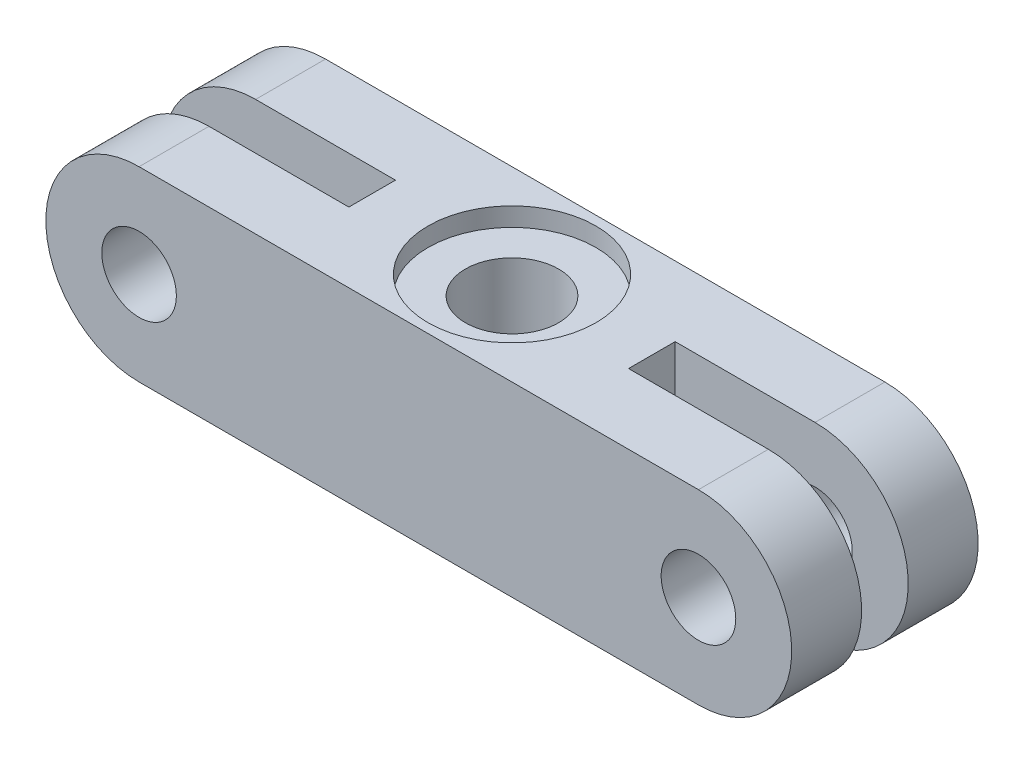
ISO-10303-21;
HEADER;
FILE_DESCRIPTION(('STEP AP214'),'2;1');
FILE_NAME('part.step','',(''),(''),'','','');
FILE_SCHEMA(('AUTOMOTIVE_DESIGN { 1 0 10303 214 1 1 1 1 }'));
ENDSEC;
DATA;
#1=APPLICATION_CONTEXT('core data for automotive mechanical design processes');
#2=APPLICATION_PROTOCOL_DEFINITION('international standard','automotive_design',2000,#1);
#3=PRODUCT_CONTEXT('',#1,'mechanical');
#4=PRODUCT('Part','Part','',(#3));
#5=PRODUCT_RELATED_PRODUCT_CATEGORY('part','',(#4));
#6=PRODUCT_DEFINITION_FORMATION('','',#4);
#7=PRODUCT_DEFINITION_CONTEXT('part definition',#1,'design');
#8=PRODUCT_DEFINITION('design','',#6,#7);
#9=PRODUCT_DEFINITION_SHAPE('','',#8);
#10=(LENGTH_UNIT() NAMED_UNIT(*) SI_UNIT(.MILLI.,.METRE.));
#11=(NAMED_UNIT(*) PLANE_ANGLE_UNIT() SI_UNIT($,.RADIAN.));
#12=(NAMED_UNIT(*) SI_UNIT($,.STERADIAN.) SOLID_ANGLE_UNIT());
#13=UNCERTAINTY_MEASURE_WITH_UNIT(LENGTH_MEASURE(1.E-05),#10,'distance_accuracy_value','');
#14=(GEOMETRIC_REPRESENTATION_CONTEXT(3) GLOBAL_UNCERTAINTY_ASSIGNED_CONTEXT((#13)) GLOBAL_UNIT_ASSIGNED_CONTEXT((#10,
#11,#12)) REPRESENTATION_CONTEXT('',''));
#15=CARTESIAN_POINT('',(0.,0.,0.));
#16=DIRECTION('',(0.,0.,1.));
#17=DIRECTION('',(1.,0.,0.));
#18=AXIS2_PLACEMENT_3D('',#15,#16,#17);
#19=CARTESIAN_POINT('',(0.,-10.,0.));
#20=DIRECTION('',(0.,1.,0.));
#21=DIRECTION('',(-1.,0.,0.));
#22=AXIS2_PLACEMENT_3D('',#19,#20,#21);
#23=CYLINDRICAL_SURFACE('',#22,5.);
#24=CARTESIAN_POINT('',(0.,-10.,0.));
#25=DIRECTION('',(0.,1.,0.));
#26=DIRECTION('',(-1.,0.,0.));
#27=AXIS2_PLACEMENT_3D('',#24,#25,#26);
#28=CIRCLE('',#27,5.);
#29=CARTESIAN_POINT('',(-5.,-10.,0.));
#30=VERTEX_POINT('',#29);
#31=EDGE_CURVE('E158',#30,#30,#28,.T.);
#32=ORIENTED_EDGE('',*,*,#31,.F.);
#33=EDGE_LOOP('',(#32));
#34=FACE_BOUND('',#33,.T.);
#35=CARTESIAN_POINT('',(0.,8.00000000000001,0.));
#36=DIRECTION('',(0.,1.,0.));
#37=DIRECTION('',(-1.,0.,0.));
#38=AXIS2_PLACEMENT_3D('',#35,#36,#37);
#39=CIRCLE('',#38,5.);
#40=CARTESIAN_POINT('',(-5.,8.00000000000001,0.));
#41=VERTEX_POINT('',#40);
#42=EDGE_CURVE('E44',#41,#41,#39,.F.);
#43=ORIENTED_EDGE('',*,*,#42,.F.);
#44=EDGE_LOOP('',(#43));
#45=FACE_BOUND('',#44,.T.);
#46=ADVANCED_FACE('F41',(#34,#45),#23,.F.);
#47=CARTESIAN_POINT('',(-30.,0.,10.));
#48=DIRECTION('',(0.,0.,-1.));
#49=DIRECTION('',(-1.,0.,0.));
#50=AXIS2_PLACEMENT_3D('',#47,#48,#49);
#51=CYLINDRICAL_SURFACE('',#50,10.);
#52=CARTESIAN_POINT('',(-30.,0.,-2.5));
#53=DIRECTION('',(0.,0.,-1.));
#54=DIRECTION('',(-1.,0.,0.));
#55=AXIS2_PLACEMENT_3D('',#52,#53,#54);
#56=CIRCLE('',#55,10.);
#57=CARTESIAN_POINT('',(-30.,-10.,-2.5));
#58=VERTEX_POINT('',#57);
#59=CARTESIAN_POINT('',(-30.,10.,-2.5));
#60=VERTEX_POINT('',#59);
#61=EDGE_CURVE('E194',#58,#60,#56,.T.);
#62=ORIENTED_EDGE('',*,*,#61,.T.);
#63=DIRECTION('',(0.,0.,-1.));
#64=VECTOR('',#63,1.);
#65=CARTESIAN_POINT('',(-30.,10.,10.));
#66=LINE('',#65,#64);
#67=CARTESIAN_POINT('',(-30.,10.,-10.));
#68=VERTEX_POINT('',#67);
#69=EDGE_CURVE('E217',#60,#68,#66,.T.);
#70=ORIENTED_EDGE('',*,*,#69,.T.);
#71=CARTESIAN_POINT('',(-30.,0.,-10.));
#72=DIRECTION('',(0.,0.,1.));
#73=DIRECTION('',(1.,0.,0.));
#74=AXIS2_PLACEMENT_3D('',#71,#72,#73);
#75=CIRCLE('',#74,10.);
#76=CARTESIAN_POINT('',(-30.,-10.,-10.));
#77=VERTEX_POINT('',#76);
#78=EDGE_CURVE('E202',#68,#77,#75,.T.);
#79=ORIENTED_EDGE('',*,*,#78,.T.);
#80=DIRECTION('',(0.,0.,-1.));
#81=VECTOR('',#80,1.);
#82=CARTESIAN_POINT('',(-30.,-10.,10.));
#83=LINE('',#82,#81);
#84=EDGE_CURVE('E49',#58,#77,#83,.T.);
#85=ORIENTED_EDGE('',*,*,#84,.F.);
#86=EDGE_LOOP('',(#62,#70,#79,#85));
#87=FACE_BOUND('',#86,.T.);
#88=ADVANCED_FACE('F283',(#87),#51,.T.);
#89=CARTESIAN_POINT('',(30.,0.,10.));
#90=DIRECTION('',(0.,0.,-1.));
#91=DIRECTION('',(-1.,0.,0.));
#92=AXIS2_PLACEMENT_3D('',#89,#90,#91);
#93=CYLINDRICAL_SURFACE('',#92,10.);
#94=DIRECTION('',(0.,0.,-1.));
#95=VECTOR('',#94,1.);
#96=CARTESIAN_POINT('',(30.,10.,10.));
#97=LINE('',#96,#95);
#98=CARTESIAN_POINT('',(30.,10.,-2.5));
#99=VERTEX_POINT('',#98);
#100=CARTESIAN_POINT('',(30.,10.,-10.));
#101=VERTEX_POINT('',#100);
#102=EDGE_CURVE('E235',#99,#101,#97,.T.);
#103=ORIENTED_EDGE('',*,*,#102,.F.);
#104=CARTESIAN_POINT('',(30.,0.,-2.5));
#105=DIRECTION('',(0.,0.,-1.));
#106=DIRECTION('',(-1.,0.,0.));
#107=AXIS2_PLACEMENT_3D('',#104,#105,#106);
#108=CIRCLE('',#107,10.);
#109=CARTESIAN_POINT('',(30.,-10.,-2.5));
#110=VERTEX_POINT('',#109);
#111=EDGE_CURVE('E189',#99,#110,#108,.T.);
#112=ORIENTED_EDGE('',*,*,#111,.T.);
#113=DIRECTION('',(0.,0.,-1.));
#114=VECTOR('',#113,1.);
#115=CARTESIAN_POINT('',(30.,-9.99999999999999,10.));
#116=LINE('',#115,#114);
#117=CARTESIAN_POINT('',(30.,-9.99999999999999,-10.));
#118=VERTEX_POINT('',#117);
#119=EDGE_CURVE('E237',#110,#118,#116,.T.);
#120=ORIENTED_EDGE('',*,*,#119,.T.);
#121=CARTESIAN_POINT('',(30.,0.,-10.));
#122=DIRECTION('',(0.,0.,1.));
#123=DIRECTION('',(1.,0.,0.));
#124=AXIS2_PLACEMENT_3D('',#121,#122,#123);
#125=CIRCLE('',#124,10.);
#126=EDGE_CURVE('E221',#118,#101,#125,.T.);
#127=ORIENTED_EDGE('',*,*,#126,.T.);
#128=EDGE_LOOP('',(#103,#112,#120,#127));
#129=FACE_BOUND('',#128,.T.);
#130=ADVANCED_FACE('F254',(#129),#93,.T.);
#131=CARTESIAN_POINT('',(-30.,0.,10.));
#132=DIRECTION('',(0.,0.,-1.));
#133=DIRECTION('',(-1.,0.,0.));
#134=AXIS2_PLACEMENT_3D('',#131,#132,#133);
#135=CYLINDRICAL_SURFACE('',#134,4.);
#136=CARTESIAN_POINT('',(-30.,0.,-2.5));
#137=DIRECTION('',(0.,0.,-1.));
#138=DIRECTION('',(-1.,0.,0.));
#139=AXIS2_PLACEMENT_3D('',#136,#137,#138);
#140=CIRCLE('',#139,4.);
#141=CARTESIAN_POINT('',(-34.,0.,-2.5));
#142=VERTEX_POINT('',#141);
#143=EDGE_CURVE('E195',#142,#142,#140,.T.);
#144=ORIENTED_EDGE('',*,*,#143,.F.);
#145=EDGE_LOOP('',(#144));
#146=FACE_BOUND('',#145,.T.);
#147=CARTESIAN_POINT('',(-30.,0.,-10.));
#148=DIRECTION('',(0.,0.,1.));
#149=DIRECTION('',(1.,0.,0.));
#150=AXIS2_PLACEMENT_3D('',#147,#148,#149);
#151=CIRCLE('',#150,4.);
#152=CARTESIAN_POINT('',(-26.,0.,-10.));
#153=VERTEX_POINT('',#152);
#154=EDGE_CURVE('E200',#153,#153,#151,.T.);
#155=ORIENTED_EDGE('',*,*,#154,.F.);
#156=EDGE_LOOP('',(#155));
#157=FACE_BOUND('',#156,.T.);
#158=ADVANCED_FACE('F253',(#146,#157),#135,.F.);
#159=CARTESIAN_POINT('',(30.,0.,10.));
#160=DIRECTION('',(0.,0.,-1.));
#161=DIRECTION('',(-1.,0.,0.));
#162=AXIS2_PLACEMENT_3D('',#159,#160,#161);
#163=CYLINDRICAL_SURFACE('',#162,4.00000000000001);
#164=CARTESIAN_POINT('',(30.,0.,-2.5));
#165=DIRECTION('',(0.,0.,-1.));
#166=DIRECTION('',(-1.,0.,0.));
#167=AXIS2_PLACEMENT_3D('',#164,#165,#166);
#168=CIRCLE('',#167,4.00000000000001);
#169=CARTESIAN_POINT('',(26.,0.,-2.5));
#170=VERTEX_POINT('',#169);
#171=EDGE_CURVE('E187',#170,#170,#168,.T.);
#172=ORIENTED_EDGE('',*,*,#171,.F.);
#173=EDGE_LOOP('',(#172));
#174=FACE_BOUND('',#173,.T.);
#175=CARTESIAN_POINT('',(30.,0.,-10.));
#176=DIRECTION('',(0.,0.,1.));
#177=DIRECTION('',(1.,0.,0.));
#178=AXIS2_PLACEMENT_3D('',#175,#176,#177);
#179=CIRCLE('',#178,4.00000000000001);
#180=CARTESIAN_POINT('',(34.,0.,-10.));
#181=VERTEX_POINT('',#180);
#182=EDGE_CURVE('E193',#181,#181,#179,.T.);
#183=ORIENTED_EDGE('',*,*,#182,.F.);
#184=EDGE_LOOP('',(#183));
#185=FACE_BOUND('',#184,.T.);
#186=ADVANCED_FACE('F255',(#174,#185),#163,.F.);
#187=CARTESIAN_POINT('',(-30.,0.,10.));
#188=DIRECTION('',(0.,0.,1.));
#189=DIRECTION('',(1.,0.,0.));
#190=AXIS2_PLACEMENT_3D('',#187,#188,#189);
#191=PLANE('',#190);
#192=CARTESIAN_POINT('',(-30.,0.,10.));
#193=DIRECTION('',(0.,0.,1.));
#194=DIRECTION('',(1.,0.,0.));
#195=AXIS2_PLACEMENT_3D('',#192,#193,#194);
#196=CIRCLE('',#195,4.);
#197=CARTESIAN_POINT('',(-26.,0.,10.));
#198=VERTEX_POINT('',#197);
#199=EDGE_CURVE('E205',#198,#198,#196,.T.);
#200=ORIENTED_EDGE('',*,*,#199,.F.);
#201=EDGE_LOOP('',(#200));
#202=FACE_BOUND('',#201,.T.);
#203=CARTESIAN_POINT('',(-30.,0.,10.));
#204=DIRECTION('',(0.,0.,1.));
#205=DIRECTION('',(1.,0.,0.));
#206=AXIS2_PLACEMENT_3D('',#203,#204,#205);
#207=CIRCLE('',#206,10.);
#208=CARTESIAN_POINT('',(-30.,10.,10.));
#209=VERTEX_POINT('',#208);
#210=CARTESIAN_POINT('',(-30.,-10.,10.));
#211=VERTEX_POINT('',#210);
#212=EDGE_CURVE('E208',#209,#211,#207,.T.);
#213=ORIENTED_EDGE('',*,*,#212,.T.);
#214=DIRECTION('',(1.,0.,0.));
#215=VECTOR('',#214,1.);
#216=CARTESIAN_POINT('',(-30.,-10.,10.));
#217=LINE('',#216,#215);
#218=CARTESIAN_POINT('',(30.,-9.99999999999999,10.));
#219=VERTEX_POINT('',#218);
#220=EDGE_CURVE('E211',#211,#219,#217,.T.);
#221=ORIENTED_EDGE('',*,*,#220,.T.);
#222=CARTESIAN_POINT('',(30.,0.,10.));
#223=DIRECTION('',(0.,0.,1.));
#224=DIRECTION('',(1.,0.,0.));
#225=AXIS2_PLACEMENT_3D('',#222,#223,#224);
#226=CIRCLE('',#225,10.);
#227=CARTESIAN_POINT('',(30.,10.,10.));
#228=VERTEX_POINT('',#227);
#229=EDGE_CURVE('E212',#219,#228,#226,.T.);
#230=ORIENTED_EDGE('',*,*,#229,.T.);
#231=DIRECTION('',(-1.,0.,0.));
#232=VECTOR('',#231,1.);
#233=CARTESIAN_POINT('',(-30.,10.,10.));
#234=LINE('',#233,#232);
#235=EDGE_CURVE('E216',#228,#209,#234,.T.);
#236=ORIENTED_EDGE('',*,*,#235,.T.);
#237=EDGE_LOOP('',(#213,#221,#230,#236));
#238=FACE_BOUND('',#237,.T.);
#239=CARTESIAN_POINT('',(30.,0.,10.));
#240=DIRECTION('',(0.,0.,1.));
#241=DIRECTION('',(1.,0.,0.));
#242=AXIS2_PLACEMENT_3D('',#239,#240,#241);
#243=CIRCLE('',#242,4.00000000000001);
#244=CARTESIAN_POINT('',(34.,0.,10.));
#245=VERTEX_POINT('',#244);
#246=EDGE_CURVE('E198',#245,#245,#243,.T.);
#247=ORIENTED_EDGE('',*,*,#246,.F.);
#248=EDGE_LOOP('',(#247));
#249=FACE_BOUND('',#248,.T.);
#250=ADVANCED_FACE('F263',(#202,#238,#249),#191,.T.);
#251=CARTESIAN_POINT('',(-30.,0.,-10.));
#252=DIRECTION('',(0.,0.,1.));
#253=DIRECTION('',(1.,0.,0.));
#254=AXIS2_PLACEMENT_3D('',#251,#252,#253);
#255=PLANE('',#254);
#256=ORIENTED_EDGE('',*,*,#78,.F.);
#257=DIRECTION('',(-1.,0.,0.));
#258=VECTOR('',#257,1.);
#259=CARTESIAN_POINT('',(-30.,10.,-10.));
#260=LINE('',#259,#258);
#261=EDGE_CURVE('E215',#101,#68,#260,.T.);
#262=ORIENTED_EDGE('',*,*,#261,.F.);
#263=ORIENTED_EDGE('',*,*,#126,.F.);
#264=DIRECTION('',(1.,0.,0.));
#265=VECTOR('',#264,1.);
#266=CARTESIAN_POINT('',(-30.,-10.,-10.));
#267=LINE('',#266,#265);
#268=EDGE_CURVE('E222',#77,#118,#267,.T.);
#269=ORIENTED_EDGE('',*,*,#268,.F.);
#270=EDGE_LOOP('',(#256,#262,#263,#269));
#271=FACE_BOUND('',#270,.T.);
#272=ORIENTED_EDGE('',*,*,#154,.T.);
#273=EDGE_LOOP('',(#272));
#274=FACE_BOUND('',#273,.T.);
#275=ORIENTED_EDGE('',*,*,#182,.T.);
#276=EDGE_LOOP('',(#275));
#277=FACE_BOUND('',#276,.T.);
#278=ADVANCED_FACE('F257',(#271,#274,#277),#255,.F.);
#279=CARTESIAN_POINT('',(-30.,10.,2.5));
#280=VERTEX_POINT('',#279);
#281=EDGE_CURVE('E228',#209,#280,#66,.T.);
#282=ORIENTED_EDGE('',*,*,#281,.T.);
#283=CARTESIAN_POINT('',(-30.,0.,2.5));
#284=DIRECTION('',(0.,0.,1.));
#285=DIRECTION('',(1.,0.,0.));
#286=AXIS2_PLACEMENT_3D('',#283,#284,#285);
#287=CIRCLE('',#286,10.);
#288=CARTESIAN_POINT('',(-30.,-10.,2.5));
#289=VERTEX_POINT('',#288);
#290=EDGE_CURVE('E67',#280,#289,#287,.T.);
#291=ORIENTED_EDGE('',*,*,#290,.T.);
#292=EDGE_CURVE('E11',#211,#289,#83,.T.);
#293=ORIENTED_EDGE('',*,*,#292,.F.);
#294=ORIENTED_EDGE('',*,*,#212,.F.);
#295=EDGE_LOOP('',(#282,#291,#293,#294));
#296=FACE_BOUND('',#295,.T.);
#297=ADVANCED_FACE('F43',(#296),#51,.T.);
#298=CARTESIAN_POINT('',(-30.,-10.,10.));
#299=DIRECTION('',(0.,1.,0.));
#300=DIRECTION('',(-1.,0.,0.));
#301=AXIS2_PLACEMENT_3D('',#298,#299,#300);
#302=PLANE('',#301);
#303=ORIENTED_EDGE('',*,*,#31,.T.);
#304=EDGE_LOOP('',(#303));
#305=FACE_BOUND('',#304,.T.);
#306=DIRECTION('',(0.,0.,-1.));
#307=VECTOR('',#306,1.);
#308=CARTESIAN_POINT('',(-15.,-10.,2.5));
#309=LINE('',#308,#307);
#310=CARTESIAN_POINT('',(-15.,-10.,2.5));
#311=VERTEX_POINT('',#310);
#312=CARTESIAN_POINT('',(-15.,-10.,-2.5));
#313=VERTEX_POINT('',#312);
#314=EDGE_CURVE('E145',#311,#313,#309,.T.);
#315=ORIENTED_EDGE('',*,*,#314,.T.);
#316=DIRECTION('',(-1.,0.,0.));
#317=VECTOR('',#316,1.);
#318=CARTESIAN_POINT('',(-15.,-10.,-2.5));
#319=LINE('',#318,#317);
#320=EDGE_CURVE('E143',#313,#58,#319,.T.);
#321=ORIENTED_EDGE('',*,*,#320,.T.);
#322=ORIENTED_EDGE('',*,*,#84,.T.);
#323=ORIENTED_EDGE('',*,*,#268,.T.);
#324=ORIENTED_EDGE('',*,*,#119,.F.);
#325=DIRECTION('',(-1.,0.,0.));
#326=VECTOR('',#325,1.);
#327=CARTESIAN_POINT('',(15.,-10.,-2.5));
#328=LINE('',#327,#326);
#329=CARTESIAN_POINT('',(15.,-10.,-2.5));
#330=VERTEX_POINT('',#329);
#331=EDGE_CURVE('E169',#110,#330,#328,.T.);
#332=ORIENTED_EDGE('',*,*,#331,.T.);
#333=DIRECTION('',(0.,0.,1.));
#334=VECTOR('',#333,1.);
#335=CARTESIAN_POINT('',(15.,-10.,2.5));
#336=LINE('',#335,#334);
#337=CARTESIAN_POINT('',(15.,-10.,2.5));
#338=VERTEX_POINT('',#337);
#339=EDGE_CURVE('E173',#330,#338,#336,.T.);
#340=ORIENTED_EDGE('',*,*,#339,.T.);
#341=DIRECTION('',(1.,0.,0.));
#342=VECTOR('',#341,1.);
#343=CARTESIAN_POINT('',(15.,-10.,2.5));
#344=LINE('',#343,#342);
#345=CARTESIAN_POINT('',(30.,-10.,2.5));
#346=VERTEX_POINT('',#345);
#347=EDGE_CURVE('E178',#338,#346,#344,.T.);
#348=ORIENTED_EDGE('',*,*,#347,.T.);
#349=EDGE_CURVE('E240',#219,#346,#116,.T.);
#350=ORIENTED_EDGE('',*,*,#349,.F.);
#351=ORIENTED_EDGE('',*,*,#220,.F.);
#352=ORIENTED_EDGE('',*,*,#292,.T.);
#353=DIRECTION('',(1.,0.,0.));
#354=VECTOR('',#353,1.);
#355=CARTESIAN_POINT('',(-15.,-10.,2.5));
#356=LINE('',#355,#354);
#357=EDGE_CURVE('E135',#289,#311,#356,.T.);
#358=ORIENTED_EDGE('',*,*,#357,.T.);
#359=EDGE_LOOP('',(#315,#321,#322,#323,#324,#332,#340,#348,#350,#351,#352,#358));
#360=FACE_BOUND('',#359,.T.);
#361=ADVANCED_FACE('F147',(#305,#360),#302,.F.);
#362=CARTESIAN_POINT('',(30.,0.,2.5));
#363=DIRECTION('',(0.,0.,1.));
#364=DIRECTION('',(1.,0.,0.));
#365=AXIS2_PLACEMENT_3D('',#362,#363,#364);
#366=CIRCLE('',#365,10.);
#367=CARTESIAN_POINT('',(30.,10.,2.5));
#368=VERTEX_POINT('',#367);
#369=EDGE_CURVE('E183',#346,#368,#366,.T.);
#370=ORIENTED_EDGE('',*,*,#369,.T.);
#371=EDGE_CURVE('E234',#228,#368,#97,.T.);
#372=ORIENTED_EDGE('',*,*,#371,.F.);
#373=ORIENTED_EDGE('',*,*,#229,.F.);
#374=ORIENTED_EDGE('',*,*,#349,.T.);
#375=EDGE_LOOP('',(#370,#372,#373,#374));
#376=FACE_BOUND('',#375,.T.);
#377=ADVANCED_FACE('F347',(#376),#93,.T.);
#378=CARTESIAN_POINT('',(-30.,10.,10.));
#379=DIRECTION('',(0.,-1.,0.));
#380=DIRECTION('',(1.,0.,0.));
#381=AXIS2_PLACEMENT_3D('',#378,#379,#380);
#382=PLANE('',#381);
#383=CARTESIAN_POINT('',(0.,10.,0.));
#384=DIRECTION('',(0.,1.,0.));
#385=DIRECTION('',(-1.,0.,0.));
#386=AXIS2_PLACEMENT_3D('',#383,#384,#385);
#387=CIRCLE('',#386,9.);
#388=CARTESIAN_POINT('',(-9.,10.,0.));
#389=VERTEX_POINT('',#388);
#390=EDGE_CURVE('E483',#389,#389,#387,.T.);
#391=ORIENTED_EDGE('',*,*,#390,.F.);
#392=EDGE_LOOP('',(#391));
#393=FACE_BOUND('',#392,.T.);
#394=ORIENTED_EDGE('',*,*,#69,.F.);
#395=DIRECTION('',(-1.,0.,0.));
#396=VECTOR('',#395,1.);
#397=CARTESIAN_POINT('',(-15.,10.,-2.5));
#398=LINE('',#397,#396);
#399=CARTESIAN_POINT('',(-15.,10.,-2.5));
#400=VERTEX_POINT('',#399);
#401=EDGE_CURVE('E155',#400,#60,#398,.T.);
#402=ORIENTED_EDGE('',*,*,#401,.F.);
#403=DIRECTION('',(0.,0.,-1.));
#404=VECTOR('',#403,1.);
#405=CARTESIAN_POINT('',(-15.,10.,2.5));
#406=LINE('',#405,#404);
#407=CARTESIAN_POINT('',(-15.,10.,2.5));
#408=VERTEX_POINT('',#407);
#409=EDGE_CURVE('E154',#408,#400,#406,.T.);
#410=ORIENTED_EDGE('',*,*,#409,.F.);
#411=DIRECTION('',(1.,0.,0.));
#412=VECTOR('',#411,1.);
#413=CARTESIAN_POINT('',(-15.,10.,2.5));
#414=LINE('',#413,#412);
#415=EDGE_CURVE('E137',#280,#408,#414,.T.);
#416=ORIENTED_EDGE('',*,*,#415,.F.);
#417=ORIENTED_EDGE('',*,*,#281,.F.);
#418=ORIENTED_EDGE('',*,*,#235,.F.);
#419=ORIENTED_EDGE('',*,*,#371,.T.);
#420=DIRECTION('',(1.,0.,0.));
#421=VECTOR('',#420,1.);
#422=CARTESIAN_POINT('',(15.,10.,2.5));
#423=LINE('',#422,#421);
#424=CARTESIAN_POINT('',(15.,10.,2.5));
#425=VERTEX_POINT('',#424);
#426=EDGE_CURVE('E174',#425,#368,#423,.T.);
#427=ORIENTED_EDGE('',*,*,#426,.F.);
#428=DIRECTION('',(0.,0.,1.));
#429=VECTOR('',#428,1.);
#430=CARTESIAN_POINT('',(15.,10.,2.5));
#431=LINE('',#430,#429);
#432=CARTESIAN_POINT('',(15.,10.,-2.5));
#433=VERTEX_POINT('',#432);
#434=EDGE_CURVE('E59',#433,#425,#431,.T.);
#435=ORIENTED_EDGE('',*,*,#434,.F.);
#436=DIRECTION('',(-1.,0.,0.));
#437=VECTOR('',#436,1.);
#438=CARTESIAN_POINT('',(15.,10.,-2.5));
#439=LINE('',#438,#437);
#440=EDGE_CURVE('E171',#99,#433,#439,.T.);
#441=ORIENTED_EDGE('',*,*,#440,.F.);
#442=ORIENTED_EDGE('',*,*,#102,.T.);
#443=ORIENTED_EDGE('',*,*,#261,.T.);
#444=EDGE_LOOP('',(#394,#402,#410,#416,#417,#418,#419,#427,#435,#441,#442,#443));
#445=FACE_BOUND('',#444,.T.);
#446=ADVANCED_FACE('F324',(#393,#445),#382,.F.);
#447=CARTESIAN_POINT('',(-30.,0.,2.5));
#448=DIRECTION('',(0.,0.,1.));
#449=DIRECTION('',(1.,0.,0.));
#450=AXIS2_PLACEMENT_3D('',#447,#448,#449);
#451=CIRCLE('',#450,4.);
#452=CARTESIAN_POINT('',(-26.,0.,2.5));
#453=VERTEX_POINT('',#452);
#454=EDGE_CURVE('E190',#453,#453,#451,.T.);
#455=ORIENTED_EDGE('',*,*,#454,.F.);
#456=EDGE_LOOP('',(#455));
#457=FACE_BOUND('',#456,.T.);
#458=ORIENTED_EDGE('',*,*,#199,.T.);
#459=EDGE_LOOP('',(#458));
#460=FACE_BOUND('',#459,.T.);
#461=ADVANCED_FACE('F260',(#457,#460),#135,.F.);
#462=CARTESIAN_POINT('',(30.,0.,2.5));
#463=DIRECTION('',(0.,0.,1.));
#464=DIRECTION('',(1.,0.,0.));
#465=AXIS2_PLACEMENT_3D('',#462,#463,#464);
#466=CIRCLE('',#465,4.00000000000001);
#467=CARTESIAN_POINT('',(34.,0.,2.49999999999999));
#468=VERTEX_POINT('',#467);
#469=EDGE_CURVE('E163',#468,#468,#466,.T.);
#470=ORIENTED_EDGE('',*,*,#469,.F.);
#471=EDGE_LOOP('',(#470));
#472=FACE_BOUND('',#471,.T.);
#473=ORIENTED_EDGE('',*,*,#246,.T.);
#474=EDGE_LOOP('',(#473));
#475=FACE_BOUND('',#474,.T.);
#476=ADVANCED_FACE('F271',(#472,#475),#163,.F.);
#477=CARTESIAN_POINT('',(15.,-10.,-2.5));
#478=DIRECTION('',(0.,0.,-1.));
#479=DIRECTION('',(-1.,0.,0.));
#480=AXIS2_PLACEMENT_3D('',#477,#478,#479);
#481=PLANE('',#480);
#482=ORIENTED_EDGE('',*,*,#171,.T.);
#483=EDGE_LOOP('',(#482));
#484=FACE_BOUND('',#483,.T.);
#485=ORIENTED_EDGE('',*,*,#440,.T.);
#486=DIRECTION('',(0.,1.,0.));
#487=VECTOR('',#486,1.);
#488=CARTESIAN_POINT('',(15.,-10.,-2.5));
#489=LINE('',#488,#487);
#490=EDGE_CURVE('E166',#330,#433,#489,.T.);
#491=ORIENTED_EDGE('',*,*,#490,.F.);
#492=ORIENTED_EDGE('',*,*,#331,.F.);
#493=ORIENTED_EDGE('',*,*,#111,.F.);
#494=EDGE_LOOP('',(#485,#491,#492,#493));
#495=FACE_BOUND('',#494,.T.);
#496=ADVANCED_FACE('F281',(#484,#495),#481,.F.);
#497=CARTESIAN_POINT('',(15.,-10.,2.5));
#498=DIRECTION('',(0.,0.,1.));
#499=DIRECTION('',(1.,0.,0.));
#500=AXIS2_PLACEMENT_3D('',#497,#498,#499);
#501=PLANE('',#500);
#502=ORIENTED_EDGE('',*,*,#469,.T.);
#503=EDGE_LOOP('',(#502));
#504=FACE_BOUND('',#503,.T.);
#505=ORIENTED_EDGE('',*,*,#369,.F.);
#506=ORIENTED_EDGE('',*,*,#347,.F.);
#507=DIRECTION('',(0.,1.,0.));
#508=VECTOR('',#507,1.);
#509=CARTESIAN_POINT('',(15.,-10.,2.5));
#510=LINE('',#509,#508);
#511=EDGE_CURVE('E167',#338,#425,#510,.T.);
#512=ORIENTED_EDGE('',*,*,#511,.T.);
#513=ORIENTED_EDGE('',*,*,#426,.T.);
#514=EDGE_LOOP('',(#505,#506,#512,#513));
#515=FACE_BOUND('',#514,.T.);
#516=ADVANCED_FACE('F309',(#504,#515),#501,.F.);
#517=CARTESIAN_POINT('',(15.,-10.,2.5));
#518=DIRECTION('',(-1.,0.,0.));
#519=DIRECTION('',(0.,-1.,0.));
#520=AXIS2_PLACEMENT_3D('',#517,#518,#519);
#521=PLANE('',#520);
#522=ORIENTED_EDGE('',*,*,#434,.T.);
#523=ORIENTED_EDGE('',*,*,#511,.F.);
#524=ORIENTED_EDGE('',*,*,#339,.F.);
#525=ORIENTED_EDGE('',*,*,#490,.T.);
#526=EDGE_LOOP('',(#522,#523,#524,#525));
#527=FACE_BOUND('',#526,.T.);
#528=ADVANCED_FACE('F302',(#527),#521,.F.);
#529=CARTESIAN_POINT('',(-15.,-10.,-2.5));
#530=DIRECTION('',(0.,0.,-1.));
#531=DIRECTION('',(-1.,0.,0.));
#532=AXIS2_PLACEMENT_3D('',#529,#530,#531);
#533=PLANE('',#532);
#534=ORIENTED_EDGE('',*,*,#143,.T.);
#535=EDGE_LOOP('',(#534));
#536=FACE_BOUND('',#535,.T.);
#537=ORIENTED_EDGE('',*,*,#61,.F.);
#538=ORIENTED_EDGE('',*,*,#320,.F.);
#539=DIRECTION('',(0.,1.,0.));
#540=VECTOR('',#539,1.);
#541=CARTESIAN_POINT('',(-15.,-10.,-2.5));
#542=LINE('',#541,#540);
#543=EDGE_CURVE('E138',#313,#400,#542,.T.);
#544=ORIENTED_EDGE('',*,*,#543,.T.);
#545=ORIENTED_EDGE('',*,*,#401,.T.);
#546=EDGE_LOOP('',(#537,#538,#544,#545));
#547=FACE_BOUND('',#546,.T.);
#548=ADVANCED_FACE('F249',(#536,#547),#533,.F.);
#549=CARTESIAN_POINT('',(-15.,-10.,2.5));
#550=DIRECTION('',(0.,0.,1.));
#551=DIRECTION('',(1.,0.,0.));
#552=AXIS2_PLACEMENT_3D('',#549,#550,#551);
#553=PLANE('',#552);
#554=ORIENTED_EDGE('',*,*,#454,.T.);
#555=EDGE_LOOP('',(#554));
#556=FACE_BOUND('',#555,.T.);
#557=ORIENTED_EDGE('',*,*,#415,.T.);
#558=DIRECTION('',(0.,1.,0.));
#559=VECTOR('',#558,1.);
#560=CARTESIAN_POINT('',(-15.,-10.,2.5));
#561=LINE('',#560,#559);
#562=EDGE_CURVE('E131',#311,#408,#561,.T.);
#563=ORIENTED_EDGE('',*,*,#562,.F.);
#564=ORIENTED_EDGE('',*,*,#357,.F.);
#565=ORIENTED_EDGE('',*,*,#290,.F.);
#566=EDGE_LOOP('',(#557,#563,#564,#565));
#567=FACE_BOUND('',#566,.T.);
#568=ADVANCED_FACE('F134',(#556,#567),#553,.F.);
#569=CARTESIAN_POINT('',(-15.,-10.,2.5));
#570=DIRECTION('',(1.,0.,0.));
#571=DIRECTION('',(0.,1.,0.));
#572=AXIS2_PLACEMENT_3D('',#569,#570,#571);
#573=PLANE('',#572);
#574=ORIENTED_EDGE('',*,*,#409,.T.);
#575=ORIENTED_EDGE('',*,*,#543,.F.);
#576=ORIENTED_EDGE('',*,*,#314,.F.);
#577=ORIENTED_EDGE('',*,*,#562,.T.);
#578=EDGE_LOOP('',(#574,#575,#576,#577));
#579=FACE_BOUND('',#578,.T.);
#580=ADVANCED_FACE('F144',(#579),#573,.F.);
#581=CARTESIAN_POINT('',(0.,8.00000000000001,0.));
#582=DIRECTION('',(0.,1.,0.));
#583=DIRECTION('',(-1.,0.,0.));
#584=AXIS2_PLACEMENT_3D('',#581,#582,#583);
#585=PLANE('',#584);
#586=CARTESIAN_POINT('',(0.,8.00000000000001,0.));
#587=DIRECTION('',(0.,1.,0.));
#588=DIRECTION('',(-1.,0.,0.));
#589=AXIS2_PLACEMENT_3D('',#586,#587,#588);
#590=CIRCLE('',#589,9.);
#591=CARTESIAN_POINT('',(-9.,8.,0.));
#592=VERTEX_POINT('',#591);
#593=EDGE_CURVE('E477',#592,#592,#590,.T.);
#594=ORIENTED_EDGE('',*,*,#593,.T.);
#595=EDGE_LOOP('',(#594));
#596=FACE_BOUND('',#595,.T.);
#597=ORIENTED_EDGE('',*,*,#42,.T.);
#598=EDGE_LOOP('',(#597));
#599=FACE_BOUND('',#598,.T.);
#600=ADVANCED_FACE('F301',(#596,#599),#585,.T.);
#601=CARTESIAN_POINT('',(0.,8.00000000000001,0.));
#602=DIRECTION('',(0.,1.,0.));
#603=DIRECTION('',(-1.,0.,0.));
#604=AXIS2_PLACEMENT_3D('',#601,#602,#603);
#605=CYLINDRICAL_SURFACE('',#604,9.);
#606=ORIENTED_EDGE('',*,*,#593,.F.);
#607=EDGE_LOOP('',(#606));
#608=FACE_BOUND('',#607,.T.);
#609=ORIENTED_EDGE('',*,*,#390,.T.);
#610=EDGE_LOOP('',(#609));
#611=FACE_BOUND('',#610,.T.);
#612=ADVANCED_FACE('F297',(#608,#611),#605,.F.);
#613=CLOSED_SHELL('',(#46,#88,#130,#158,#186,#250,#278,#297,#361,#377,#446,#461,#476,#496,#516,
#528,#548,#568,#580,#600,#612));
#614=MANIFOLD_SOLID_BREP('B2',#613);
#615=ADVANCED_BREP_SHAPE_REPRESENTATION('',(#18,#614),#14);
#616=SHAPE_DEFINITION_REPRESENTATION(#9,#615);
ENDSEC;
END-ISO-10303-21;
